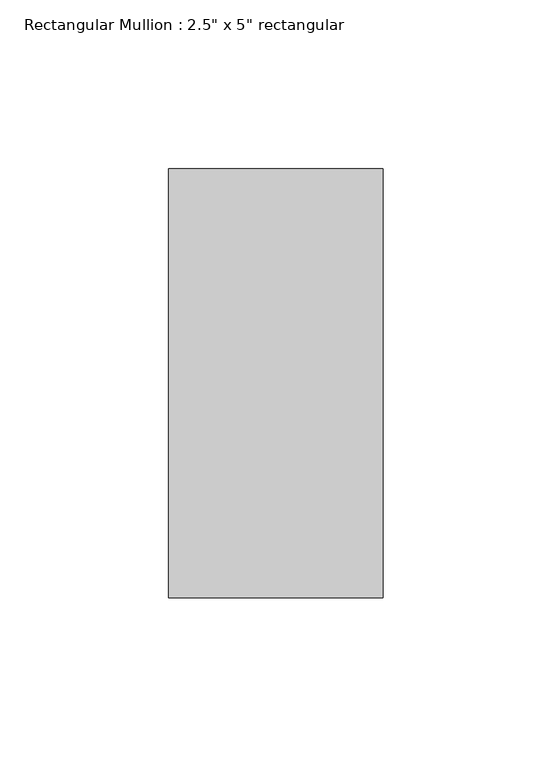
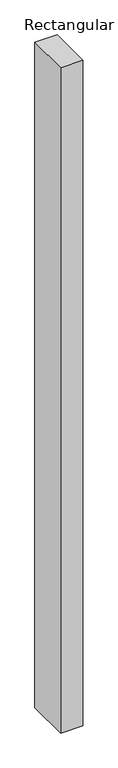
"""IFC4 building model written with IfcOpenShell, lengths in millimetres: member geometry."""

from ifc_helpers import new_model, si_unit, frame, origin, place, context, project, spatial, polyline, outline, extrude, source, transform, mapped, element, save


def member_2710255a(model_context):
    return source(origin(), model_context, "Body", "SweptSolid", [
        extrude(outline(polyline([(0.0, 63.5), (0.0, -63.5), (-63.5, -63.5), (-63.5, 63.5), (0.0, 63.5)])), frame((0.0, 0.0, -2009.4971724), z_axis=(0.0, 0.0, 1.0), x_axis=(1.0, 0.0, 0.0)), (0.0, 0.0, 1.0), 2009.4971724),
    ])


if __name__ == "__main__":
    model = new_model("IFC4")
    model_context = context("Model", 3, world=origin())
    ifc_project = project(units=[si_unit("LENGTHUNIT", "METRE", prefix="MILLI")], contexts=[model_context])
    site = spatial("IfcSite", under=ifc_project)
    building = spatial("IfcBuilding", under=site)
    placement = place(None, origin())
    member_shape = member_2710255a(model_context)
    element("IfcMember", 1, ObjectType="Rectangular Mullion : 2.5\" x 5\" rectangular", at=placement, inside=building, context=model_context, shape_type="MappedRepresentation", body=[
        mapped(member_shape, transform((0.0, 0.0, 0.0), x_axis=(1.0, 0.0, 0.0), y_axis=(0.0, 1.0, 0.0), z_axis=(0.0, 0.0, 1.0))),
    ])
    save(model, "model.ifc")

# Revit data of these elements
# Type "Rectangular Mullion : 2.5\" x 5\" rectangular"
#   built-in parameter 1007304 = 0.416667 (stored number, unit not read)
#   built-in parameter 1007301 = 0.104167 (stored number, unit not read)
#   built-in parameter 1007300 = 0.104167 (stored number, unit not read)
# Element 1 (IfcMember, "Rectangular Mullion : 2.5\" x 5\" rectangular")
#   Materials on its faces: "Aluminum"
# Materials
#   "Aluminum": class "Metal", colour RGB 247 247 247, transparency 0, Description = "Aluminum 6061", Cost = 0
